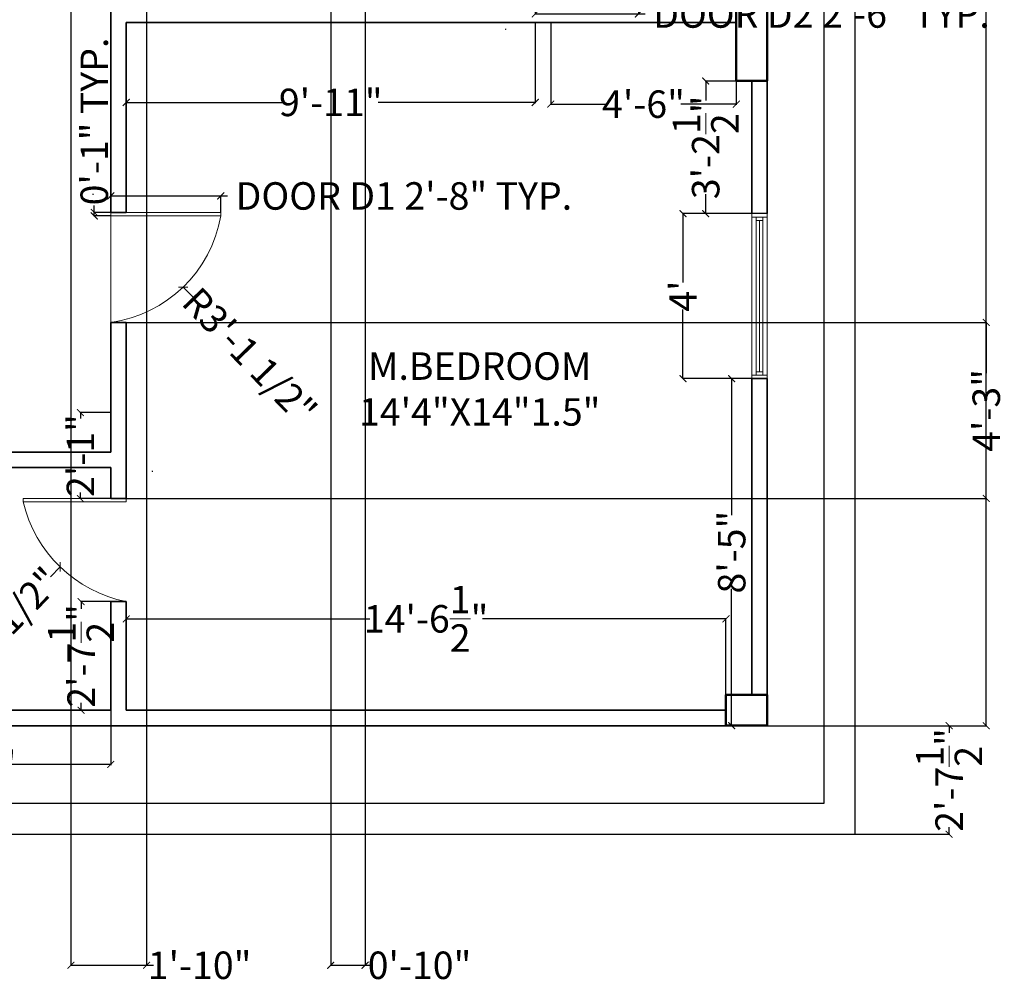
# Model space of a CAD drawing. Units: inches. Extents: x 490 to 1091, y 501 to 1322.
# Tile 2 of 5: x 804 to 1091, y 508 to 788. Entities that reach past the tile are written whole.
import ezdxf

# ---------------------------------------------------------------- set-up
doc = ezdxf.new("R2010")
doc.units = ezdxf.units.IN
doc.header["$MEASUREMENT"] = 0
for name, color, linetype, lineweight in [('A-ANNO-DIMS', 2, 'Continuous', 18), ('A-AREA-IDEN', 7, 'Continuous', 25), ('A-COLS', 12, 'Continuous', 50), ('A-DOOR', 3, 'Continuous', 20), ('A-GLAZ', 4, 'Continuous', 18), ('A-WALL', 7, 'Continuous', 35), ('C-PROP', 8, 'Continuous', 25)]:
    doc.layers.add(name, color=color, linetype=linetype, lineweight=lineweight)
doc.styles.get("Standard").update_dxf_attribs({"font": 'arial.ttf'})
doc.dimstyles.get("Standard").update_dxf_attribs({"dimtxt": 8, "dimasz": 2, "dimexe": 0.18, "dimexo": 0.0625, "dimgap": 0.09, "dimtad": 0, "dimdec": 1, "dimzin": 0, "dimdsep": 46, "dimlunit": 4, "dimtxsty": 'Standard', "dimblk": 'ARCHTICK', "dimcen": 0.09, "dimadec": 0, "dimazin": 0, "dimtfac": 1, "dimtdec": 1, "dimtofl": 0, "dimtmove": 0, "dimatfit": 3, "dimldrblk": 'ARCHTICK', "dimfxl": 1, "dimtolj": 1, "dimtzin": 0, "dimarcsym": 0})

# ---------------------------------------------------------------- blocks, each defined once
blk = doc.blocks.new('jcjg  bmvh')
for p, q in [((1232.66, 1066.6), (1223.66, 1066.6)), ((1223.66, 1066.6), (1223.66, 1042.6)), ((1232.66, 1042.6), (1232.66, 1066.6)), ((1223.66, 1042.6), (1232.66, 1042.6))]:
    blk.add_line(p, q)
blk = doc.blocks.new('bnfgfhvhm')
for p, q in [((1106.43, 1203.63), (1115.43, 1203.63)), ((1106.43, 1191.63), (1106.43, 1203.63)), ((1115.43, 1203.63), (1115.43, 1191.63)), ((1115.43, 1191.63), (1106.43, 1191.63))]:
    blk.add_line(p, q)
blk = doc.blocks.new('_ArchTick')
at = {"color": 0, "linetype": 'ByBlock', "const_width": 0.15}
blk.add_lwpolyline([(-0.5, -0.5), (0.5, 0.5)], dxfattribs=at)
blk = doc.blocks.new('*D16')
at = {"layer": 'A-ANNO-DIMS', "color": 0, "lineweight": -2, "transparency": 16777216}
for p, q in [((830.61, 618.58), (821.86, 618.58)), ((822.04, 618.58), (822.04, 616.49)), ((822.04, 586.98), (822.04, 589.08)), ((830.61, 586.98), (821.86, 586.98))]:
    blk.add_line(p, q, dxfattribs=at)
at = {"layer": 'Defpoints', "color": 0, "transparency": 16777216}
for p in [(822.04, 618.58), (830.67, 618.58), (830.67, 586.98)]:
    blk.add_point(p, dxfattribs=at)
at = {"layer": 'A-ANNO-DIMS', "color": 0, "lineweight": -2, "transparency": 16777216, "xscale": 2, "yscale": 2, "zscale": 2}
for p, rotation in [((822.04, 618.58), 90), ((822.04, 586.98), 270)]:
    blk.add_blockref('_ArchTick', p, dxfattribs=dict(at, rotation=rotation))
at = {"layer": 'A-ANNO-DIMS', "color": 0, "transparency": 16777216, "insert": (822.04, 602.78), "char_height": 8, "attachment_point": 5, "rotation": 90}
blk.add_mtext('\\A1;2\'-7{\\H1x;\\S1/2;}"', dxfattribs=at)
blk = doc.blocks.new('*D17')
at = {"layer": 'A-ANNO-DIMS', "color": 0, "lineweight": -2, "transparency": 16777216}
for p, q in [((830.61, 673.58), (821.66, 673.58)), ((821.84, 673.58), (821.84, 671.88)), ((830.61, 648.58), (821.66, 648.58)), ((821.84, 648.58), (821.84, 650.29))]:
    blk.add_line(p, q, dxfattribs=at)
at = {"layer": 'Defpoints', "color": 0, "transparency": 16777216}
for p in [(830.67, 673.58), (821.84, 648.58), (830.67, 648.58)]:
    blk.add_point(p, dxfattribs=at)
at = {"layer": 'A-ANNO-DIMS', "color": 0, "lineweight": -2, "transparency": 16777216, "xscale": 2, "yscale": 2, "zscale": 2}
for p, rotation in [((821.84, 673.58), 90), ((821.84, 648.58), 270)]:
    blk.add_blockref('_ArchTick', p, dxfattribs=dict(at, rotation=rotation))
at = {"layer": 'A-ANNO-DIMS', "color": 0, "transparency": 16777216, "insert": (821.84, 661.08), "char_height": 8, "attachment_point": 5, "rotation": 90}
blk.add_mtext('\\A1;2\'-1"', dxfattribs=at)
blk = doc.blocks.new('*D18')
at = {"layer": 'A-ANNO-DIMS', "color": 0, "lineweight": -2, "transparency": 16777216}
for p, q in [((751.67, 586.92), (751.67, 571.01)), ((830.67, 586.92), (830.67, 571.01)), ((751.67, 571.19), (780.42, 571.19)), ((830.67, 571.19), (801.91, 571.19))]:
    blk.add_line(p, q, dxfattribs=at)
at = {"layer": 'Defpoints', "color": 0, "transparency": 16777216}
for p in [(751.67, 586.98), (830.67, 586.98), (751.67, 571.19)]:
    blk.add_point(p, dxfattribs=at)
at = {"layer": 'A-ANNO-DIMS', "color": 0, "lineweight": -2, "transparency": 16777216, "xscale": 2, "yscale": 2, "zscale": 2, "rotation": 180}
blk.add_blockref('_ArchTick', (751.67, 571.19), dxfattribs=at)
at = {"layer": 'A-ANNO-DIMS', "color": 0, "lineweight": -2, "transparency": 16777216, "xscale": 2, "yscale": 2, "zscale": 2}
blk.add_blockref('_ArchTick', (830.67, 571.19), dxfattribs=at)
at = {"layer": 'A-ANNO-DIMS', "color": 0, "transparency": 16777216, "insert": (791.17, 571.19), "char_height": 8, "attachment_point": 5}
blk.add_mtext('\\A1;6\'-7"', dxfattribs=at)
blk = doc.blocks.new('mhjyhjykmjk')
for p, q in [((1017.17, 683.48), (1017.17, 731.48)), ((1017.17, 731.48), (1021.67, 731.48)), ((1021.67, 731.48), (1021.67, 683.48)), ((1017.17, 730.48), (1021.67, 730.48)), ((1018.42, 730.48), (1018.42, 684.48)), ((1018.42, 729.48), (1020.42, 729.48)), ((1019.42, 729.48), (1019.42, 685.48)), ((1020.42, 730.48), (1020.42, 684.48)), ((1020.42, 685.48), (1018.42, 685.48)), ((1021.67, 684.48), (1017.17, 684.48)), ((1021.67, 683.48), (1017.17, 683.48))]:
    blk.add_line(p, q)
at = {"layer": 'Defpoints'}
for p, q in [((1021.67, 731.48), (1017.17, 731.48)), ((1017.17, 683.48), (1021.67, 683.48))]:
    blk.add_line(p, q, dxfattribs=at)
blk = doc.blocks.new('*D37')
at = {"layer": 'A-ANNO-DIMS', "color": 0, "lineweight": -2, "transparency": 16777216}
for p, q in [((1021.73, 582.48), (1074.78, 582.48)), ((1074.6, 582.48), (1074.6, 580.39)), ((1074.6, 550.88), (1074.6, 552.98)), ((1047.33, 550.88), (1074.78, 550.88))]:
    blk.add_line(p, q, dxfattribs=at)
at = {"layer": 'Defpoints', "color": 0, "transparency": 16777216}
for p in [(1021.67, 582.48), (1047.27, 550.88), (1074.6, 550.88)]:
    blk.add_point(p, dxfattribs=at)
at = {"layer": 'A-ANNO-DIMS', "color": 0, "lineweight": -2, "transparency": 16777216, "xscale": 2, "yscale": 2, "zscale": 2}
for p, rotation in [((1074.6, 582.48), 90), ((1074.6, 550.88), 270)]:
    blk.add_blockref('_ArchTick', p, dxfattribs=dict(at, rotation=rotation))
at = {"layer": 'A-ANNO-DIMS', "color": 0, "transparency": 16777216, "insert": (1074.6, 566.68), "char_height": 8, "attachment_point": 5, "rotation": 90}
blk.add_mtext('\\A1;2\'-7{\\H1x;\\S1/2;}"', dxfattribs=at)
blk = doc.blocks.new('*D40')
at = {"layer": 'A-ANNO-DIMS', "color": 0, "lineweight": -2, "transparency": 16777216}
for p, q in [((835.17, 787.02), (835.17, 763.67)), ((954.17, 787.02), (954.17, 763.67)), ((835.17, 763.85), (880.84, 763.85)), ((954.17, 763.85), (908.5, 763.85))]:
    blk.add_line(p, q, dxfattribs=at)
at = {"layer": 'Defpoints', "color": 0, "transparency": 16777216}
for p in [(835.17, 787.08), (954.17, 787.08), (835.17, 763.85)]:
    blk.add_point(p, dxfattribs=at)
at = {"layer": 'A-ANNO-DIMS', "color": 0, "lineweight": -2, "transparency": 16777216, "xscale": 2, "yscale": 2, "zscale": 2, "rotation": 180}
blk.add_blockref('_ArchTick', (835.17, 763.85), dxfattribs=at)
at = {"layer": 'A-ANNO-DIMS', "color": 0, "lineweight": -2, "transparency": 16777216, "xscale": 2, "yscale": 2, "zscale": 2}
blk.add_blockref('_ArchTick', (954.17, 763.85), dxfattribs=at)
at = {"layer": 'A-ANNO-DIMS', "color": 0, "transparency": 16777216, "insert": (894.67, 763.85), "char_height": 8, "attachment_point": 5}
blk.add_mtext('\\A1;9\'-11"', dxfattribs=at)
blk = doc.blocks.new('*D41')
at = {"layer": 'A-ANNO-DIMS', "color": 0, "lineweight": -2, "transparency": 16777216}
for p, q in [((958.67, 787.02), (958.67, 763.17)), ((1012.67, 787.02), (1012.67, 763.17)), ((958.67, 763.35), (974.79, 763.35)), ((1012.67, 763.35), (996.55, 763.35))]:
    blk.add_line(p, q, dxfattribs=at)
at = {"layer": 'Defpoints', "color": 0, "transparency": 16777216}
for p in [(958.67, 787.08), (1012.67, 787.08), (1012.67, 763.35)]:
    blk.add_point(p, dxfattribs=at)
at = {"layer": 'A-ANNO-DIMS', "color": 0, "lineweight": -2, "transparency": 16777216, "xscale": 2, "yscale": 2, "zscale": 2, "rotation": 180}
blk.add_blockref('_ArchTick', (958.67, 763.35), dxfattribs=at)
at = {"layer": 'A-ANNO-DIMS', "color": 0, "lineweight": -2, "transparency": 16777216, "xscale": 2, "yscale": 2, "zscale": 2}
blk.add_blockref('_ArchTick', (1012.67, 763.35), dxfattribs=at)
at = {"layer": 'A-ANNO-DIMS', "color": 0, "transparency": 16777216, "insert": (985.67, 763.35), "char_height": 8, "attachment_point": 5}
blk.add_mtext('\\A1;4\'-6"', dxfattribs=at)
blk = doc.blocks.new('*D42')
at = {"layer": 'A-ANNO-DIMS', "color": 0, "lineweight": -2, "transparency": 16777216}
for p, q in [((1021.61, 683.48), (1011.14, 683.48)), ((1011.32, 683.48), (1011.32, 643.71)), ((1011.32, 582.48), (1011.32, 622.26)), ((1021.61, 582.48), (1011.14, 582.48))]:
    blk.add_line(p, q, dxfattribs=at)
at = {"layer": 'Defpoints', "color": 0, "transparency": 16777216}
for p in [(1021.67, 683.48), (1011.32, 582.48), (1021.67, 582.48)]:
    blk.add_point(p, dxfattribs=at)
at = {"layer": 'A-ANNO-DIMS', "color": 0, "lineweight": -2, "transparency": 16777216, "xscale": 2, "yscale": 2, "zscale": 2}
for p, rotation in [((1011.32, 683.48), 90), ((1011.32, 582.48), 270)]:
    blk.add_blockref('_ArchTick', p, dxfattribs=dict(at, rotation=rotation))
at = {"layer": 'A-ANNO-DIMS', "color": 0, "transparency": 16777216, "insert": (1011.32, 632.98), "char_height": 8, "attachment_point": 5, "rotation": 90}
blk.add_mtext('\\A1;8\'-5"', dxfattribs=at)
blk = doc.blocks.new('*D43')
at = {"layer": 'A-ANNO-DIMS', "color": 0, "lineweight": -2, "transparency": 16777216}
for p, q in [((1017.11, 731.48), (996.97, 731.48)), ((997.15, 731.48), (997.15, 711.42)), ((997.15, 683.48), (997.15, 703.55)), ((1017.11, 683.48), (996.97, 683.48))]:
    blk.add_line(p, q, dxfattribs=at)
at = {"layer": 'Defpoints', "color": 0, "transparency": 16777216}
for p in [(997.15, 731.48), (1017.17, 731.48), (1017.17, 683.48)]:
    blk.add_point(p, dxfattribs=at)
at = {"layer": 'A-ANNO-DIMS', "color": 0, "lineweight": -2, "transparency": 16777216, "xscale": 2, "yscale": 2, "zscale": 2}
for p, rotation in [((997.15, 731.48), 90), ((997.15, 683.48), 270)]:
    blk.add_blockref('_ArchTick', p, dxfattribs=dict(at, rotation=rotation))
at = {"layer": 'A-ANNO-DIMS', "color": 0, "transparency": 16777216, "insert": (997.15, 707.48), "char_height": 8, "attachment_point": 5, "rotation": 90}
blk.add_mtext("\\A1;4'", dxfattribs=at)
blk = doc.blocks.new('*D44')
at = {"layer": 'A-ANNO-DIMS', "color": 0, "lineweight": -2, "transparency": 16777216}
for p, q in [((1017.11, 770.08), (1003.58, 770.08)), ((1003.76, 770.08), (1003.76, 764.42)), ((1003.76, 731.48), (1003.76, 737.15)), ((1017.11, 731.48), (1003.58, 731.48))]:
    blk.add_line(p, q, dxfattribs=at)
at = {"layer": 'Defpoints', "color": 0, "transparency": 16777216}
for p in [(1017.17, 770.08), (1003.76, 731.48), (1017.17, 731.48)]:
    blk.add_point(p, dxfattribs=at)
at = {"layer": 'A-ANNO-DIMS', "color": 0, "lineweight": -2, "transparency": 16777216, "xscale": 2, "yscale": 2, "zscale": 2}
for p, rotation in [((1003.76, 770.08), 90), ((1003.76, 731.48), 270)]:
    blk.add_blockref('_ArchTick', p, dxfattribs=dict(at, rotation=rotation))
at = {"layer": 'A-ANNO-DIMS', "color": 0, "transparency": 16777216, "insert": (1003.76, 750.78), "char_height": 8, "attachment_point": 5, "rotation": 90}
blk.add_mtext('\\A1;3\'-2{\\H1x;\\S1/2;}"', dxfattribs=at)
blk = doc.blocks.new('*D45')
at = {"layer": 'A-ANNO-DIMS', "color": 0, "lineweight": -2, "transparency": 16777216}
for p, q in [((835.17, 587.05), (835.17, 613.75)), ((835.17, 613.57), (906.05, 613.57)), ((1009.67, 613.57), (938.79, 613.57)), ((1009.67, 587.05), (1009.67, 613.75))]:
    blk.add_line(p, q, dxfattribs=at)
at = {"layer": 'Defpoints', "color": 0, "transparency": 16777216}
for p in [(1009.67, 613.57), (835.17, 586.98), (1009.67, 586.98)]:
    blk.add_point(p, dxfattribs=at)
at = {"layer": 'A-ANNO-DIMS', "color": 0, "lineweight": -2, "transparency": 16777216, "xscale": 2, "yscale": 2, "zscale": 2, "rotation": 180}
blk.add_blockref('_ArchTick', (835.17, 613.57), dxfattribs=at)
at = {"layer": 'A-ANNO-DIMS', "color": 0, "lineweight": -2, "transparency": 16777216, "xscale": 2, "yscale": 2, "zscale": 2}
blk.add_blockref('_ArchTick', (1009.67, 613.57), dxfattribs=at)
at = {"layer": 'A-ANNO-DIMS', "color": 0, "transparency": 16777216, "insert": (922.42, 613.57), "char_height": 8, "attachment_point": 5}
blk.add_mtext('\\A1;14\'-6{\\H1x;\\S1/2;}"', dxfattribs=at)
blk = doc.blocks.new('DOOR-LEAF-32IN')
for p, q in [((-32, -1), (-32, 0)), ((-32, 0), (0, 0)), ((0, 0), (0, -1)), ((0, -1), (-32, -1))]:
    blk.add_line(p, q)
blk = doc.blocks.new('DOOR-LEAF-30IN')
for p, q in [((0, 0), (0, 1)), ((0, 1), (30, 1)), ((30, 0), (0, 0)), ((30, 1), (30, 0))]:
    blk.add_line(p, q)
blk = doc.blocks.new('*D54')
at = {"layer": 'A-ANNO-DIMS', "color": 0, "lineweight": -2, "transparency": 16777216}
for p, q in [((830.67, 731.9), (830.67, 736.81)), ((830.67, 736.63), (862.67, 736.63)), ((862.67, 731.9), (862.67, 736.81)), ((862.67, 736.63), (864.67, 736.63))]:
    blk.add_line(p, q, dxfattribs=at)
at = {"layer": 'Defpoints', "color": 0, "transparency": 16777216}
for p in [(862.67, 736.63), (830.67, 731.83), (862.67, 731.83)]:
    blk.add_point(p, dxfattribs=at)
at = {"layer": 'A-ANNO-DIMS', "color": 0, "lineweight": -2, "transparency": 16777216, "xscale": 2, "yscale": 2, "zscale": 2, "rotation": 180}
blk.add_blockref('_ArchTick', (830.67, 736.63), dxfattribs=at)
at = {"layer": 'A-ANNO-DIMS', "color": 0, "lineweight": -2, "transparency": 16777216, "xscale": 2, "yscale": 2, "zscale": 2}
blk.add_blockref('_ArchTick', (862.67, 736.63), dxfattribs=at)
at = {"layer": 'A-ANNO-DIMS', "color": 0, "transparency": 16777216, "insert": (915.95, 736.63), "char_height": 8, "attachment_point": 5}
blk.add_mtext('\\A1;DOOR D1 2\'-8" TYP.', dxfattribs=at)
blk = doc.blocks.new('*D55')
at = {"layer": 'A-ANNO-DIMS', "color": 0, "lineweight": -2, "transparency": 16777216}
for p, q in [((825.87, 731.83), (825.87, 733.83)), ((830.61, 731.83), (825.69, 731.83)), ((830.61, 730.83), (825.69, 730.83)), ((825.87, 730.83), (825.87, 731.83))]:
    blk.add_line(p, q, dxfattribs=at)
at = {"layer": 'Defpoints', "color": 0, "transparency": 16777216}
for p in [(825.87, 731.83), (830.67, 731.83), (830.67, 730.83)]:
    blk.add_point(p, dxfattribs=at)
at = {"layer": 'A-ANNO-DIMS', "color": 0, "lineweight": -2, "transparency": 16777216, "xscale": 2, "yscale": 2, "zscale": 2}
for p, rotation in [((825.87, 731.83), 90), ((825.87, 730.83), 270)]:
    blk.add_blockref('_ArchTick', p, dxfattribs=dict(at, rotation=rotation))
at = {"layer": 'A-ANNO-DIMS', "color": 0, "transparency": 16777216, "insert": (825.87, 758.3), "char_height": 8, "attachment_point": 5, "rotation": 90}
blk.add_mtext('\\A1;0\'-1" TYP.', dxfattribs=at)
blk = doc.blocks.new('*D56')
at = {"layer": 'A-ANNO-DIMS', "color": 0, "lineweight": -2, "transparency": 16777216}
for p, q in [((954.17, 794.02), (954.17, 789.4)), ((984.17, 794.02), (984.17, 789.4)), ((954.17, 789.58), (984.17, 789.58)), ((984.17, 789.58), (986.17, 789.58))]:
    blk.add_line(p, q, dxfattribs=at)
at = {"layer": 'Defpoints', "color": 0, "transparency": 16777216}
for p in [(954.17, 794.08), (984.17, 794.08), (984.17, 789.58)]:
    blk.add_point(p, dxfattribs=at)
at = {"layer": 'A-ANNO-DIMS', "color": 0, "lineweight": -2, "transparency": 16777216, "xscale": 2, "yscale": 2, "zscale": 2, "rotation": 180}
blk.add_blockref('_ArchTick', (954.17, 789.58), dxfattribs=at)
at = {"layer": 'A-ANNO-DIMS', "color": 0, "lineweight": -2, "transparency": 16777216, "xscale": 2, "yscale": 2, "zscale": 2}
blk.add_blockref('_ArchTick', (984.17, 789.58), dxfattribs=at)
at = {"layer": 'A-ANNO-DIMS', "color": 0, "transparency": 16777216, "insert": (1037.45, 789.58), "char_height": 8, "attachment_point": 5}
blk.add_mtext('\\A1;DOOR D2 2\'-6" TYP.', dxfattribs=at)
blk = doc.blocks.new('*D65')
at = {"layer": 'A-ANNO-DIMS', "color": 0, "lineweight": -2, "transparency": 16777216}
for p, q in [((1021.73, 1227.28), (1085.58, 1227.28)), ((1085.4, 1227.28), (1085.4, 918.72)), ((1085.4, 582.48), (1085.4, 891.05)), ((1021.73, 582.48), (1085.58, 582.48))]:
    blk.add_line(p, q, dxfattribs=at)
at = {"layer": 'Defpoints', "color": 0, "transparency": 16777216}
for p in [(1021.67, 1227.28), (1085.4, 1227.28), (1021.67, 582.48)]:
    blk.add_point(p, dxfattribs=at)
at = {"layer": 'A-ANNO-DIMS', "color": 0, "lineweight": -2, "transparency": 16777216, "xscale": 2, "yscale": 2, "zscale": 2}
for p, rotation in [((1085.4, 1227.28), 90), ((1085.4, 582.48), 270)]:
    blk.add_blockref('_ArchTick', p, dxfattribs=dict(at, rotation=rotation))
at = {"layer": 'A-ANNO-DIMS', "color": 0, "transparency": 16777216, "insert": (1085.4, 904.88), "char_height": 8, "attachment_point": 5, "rotation": 90}
blk.add_mtext('\\A1;53\'-9"', dxfattribs=at)
blk = doc.blocks.new('*D69')
at = {"layer": 'A-ANNO-DIMS', "color": 0, "lineweight": -2, "transparency": 16777216}
for p, q in [((894.67, 1182.97), (894.67, 512.57)), ((904.67, 1182.97), (904.67, 512.57)), ((894.67, 512.75), (904.67, 512.75)), ((904.67, 512.75), (906.67, 512.75))]:
    blk.add_line(p, q, dxfattribs=at)
at = {"layer": 'Defpoints', "color": 0, "transparency": 16777216}
for p in [(894.67, 1183.03), (904.67, 1183.03), (904.67, 512.75)]:
    blk.add_point(p, dxfattribs=at)
at = {"layer": 'A-ANNO-DIMS', "color": 0, "lineweight": -2, "transparency": 16777216, "xscale": 2, "yscale": 2, "zscale": 2, "rotation": 180}
blk.add_blockref('_ArchTick', (894.67, 512.75), dxfattribs=at)
at = {"layer": 'A-ANNO-DIMS', "color": 0, "lineweight": -2, "transparency": 16777216, "xscale": 2, "yscale": 2, "zscale": 2}
blk.add_blockref('_ArchTick', (904.67, 512.75), dxfattribs=at)
at = {"layer": 'A-ANNO-DIMS', "color": 0, "transparency": 16777216, "insert": (920.5, 512.75), "char_height": 8, "attachment_point": 5}
blk.add_mtext('\\A1;0\'-10"', dxfattribs=at)
blk = doc.blocks.new('*D71')
at = {"layer": 'A-ANNO-DIMS', "color": 0, "lineweight": -2, "transparency": 16777216}
for p, q in [((819.07, 1134.22), (819.07, 512.57)), ((841.07, 1134.22), (841.07, 512.57)), ((819.07, 512.75), (841.07, 512.75)), ((841.07, 512.75), (843.07, 512.75))]:
    blk.add_line(p, q, dxfattribs=at)
at = {"layer": 'Defpoints', "color": 0, "transparency": 16777216}
for p in [(819.07, 1134.28), (841.07, 1134.28), (841.07, 512.75)]:
    blk.add_point(p, dxfattribs=at)
at = {"layer": 'A-ANNO-DIMS', "color": 0, "lineweight": -2, "transparency": 16777216, "xscale": 2, "yscale": 2, "zscale": 2, "rotation": 180}
blk.add_blockref('_ArchTick', (819.07, 512.75), dxfattribs=at)
at = {"layer": 'A-ANNO-DIMS', "color": 0, "lineweight": -2, "transparency": 16777216, "xscale": 2, "yscale": 2, "zscale": 2}
blk.add_blockref('_ArchTick', (841.07, 512.75), dxfattribs=at)
at = {"layer": 'A-ANNO-DIMS', "color": 0, "transparency": 16777216, "insert": (856.52, 512.75), "char_height": 8, "attachment_point": 5}
blk.add_mtext('\\A1;1\'-10"', dxfattribs=at)
blk = doc.blocks.new('*D80')
at = {"layer": 'A-ANNO-DIMS', "color": 0, "lineweight": -2, "transparency": 16777216}
for p, q in [((830.73, 699.83), (1085.58, 699.83)), ((1085.4, 699.83), (1085.4, 685.09)), ((1085.4, 648.58), (1085.4, 663.32)), ((830.73, 648.58), (1085.58, 648.58))]:
    blk.add_line(p, q, dxfattribs=at)
at = {"layer": 'Defpoints', "color": 0, "transparency": 16777216}
for p in [(830.67, 699.83), (1085.4, 699.83), (830.67, 648.58)]:
    blk.add_point(p, dxfattribs=at)
at = {"layer": 'A-ANNO-DIMS', "color": 0, "lineweight": -2, "transparency": 16777216, "xscale": 2, "yscale": 2, "zscale": 2}
for p, rotation in [((1085.4, 699.83), 90), ((1085.4, 648.58), 270)]:
    blk.add_blockref('_ArchTick', p, dxfattribs=dict(at, rotation=rotation))
at = {"layer": 'A-ANNO-DIMS', "color": 0, "transparency": 16777216, "insert": (1085.4, 674.21), "char_height": 8, "attachment_point": 5, "rotation": 90}
blk.add_mtext('\\A1;4\'-3"', dxfattribs=at)
blk = doc.blocks.new('*D82')
at = {"layer": 'A-ANNO-DIMS', "color": 0, "lineweight": -2, "transparency": 16777216}
for p, q in [((979.77, 820.56), (973.27, 813.82)), ((945.48, 785.17), (945.66, 785.17)), ((945.57, 785.08), (945.57, 785.26))]:
    blk.add_line(p, q, dxfattribs=at)
at = {"layer": 'Defpoints', "color": 0, "transparency": 16777216}
for p in [(973.27, 813.82), (945.57, 785.17)]:
    blk.add_point(p, dxfattribs=at)
at = {"layer": 'A-ANNO-DIMS', "color": 0, "lineweight": -2, "transparency": 16777216, "xscale": 2, "yscale": 2, "zscale": 2, "rotation": 225.9717309641953}
blk.add_blockref('_ArchTick', (973.27, 813.82), dxfattribs=at)
at = {"layer": 'A-ANNO-DIMS', "color": 0, "transparency": 16777216, "insert": (989.89, 831.02), "char_height": 8, "attachment_point": 5, "rotation": 45.9717}
blk.add_mtext('\\A1;R3\'-4"', dxfattribs=at)
blk = doc.blocks.new('*D84')
at = {"layer": 'A-ANNO-DIMS', "color": 0, "lineweight": -2, "transparency": 16777216}
for p, q in [((842.73, 656.51), (842.91, 656.51)), ((842.82, 656.42), (842.82, 656.6)), ((813.15, 625.82), (815.93, 628.69))]:
    blk.add_line(p, q, dxfattribs=at)
at = {"layer": 'Defpoints', "color": 0, "transparency": 16777216}
for p in [(842.82, 656.51), (815.93, 628.69)]:
    blk.add_point(p, dxfattribs=at)
at = {"layer": 'A-ANNO-DIMS', "color": 0, "lineweight": -2, "transparency": 16777216, "xscale": 2, "yscale": 2, "zscale": 2, "rotation": 45.97167705914391}
blk.add_blockref('_ArchTick', (815.93, 628.69), dxfattribs=at)
at = {"layer": 'A-ANNO-DIMS', "color": 0, "transparency": 16777216, "insert": (796.55, 608.65), "char_height": 8, "attachment_point": 5, "rotation": 45.9717}
blk.add_mtext('\\A1;R3\'-2 1/2"', dxfattribs=at)
blk = doc.blocks.new('*D85')
at = {"layer": 'A-ANNO-DIMS', "color": 0, "lineweight": -2, "transparency": 16777216}
for p, q in [((825.42, 737.17), (825.6, 737.17)), ((825.51, 737.08), (825.51, 737.26)), ((854.52, 707.23), (851.74, 710.1))]:
    blk.add_line(p, q, dxfattribs=at)
at = {"layer": 'Defpoints', "color": 0, "transparency": 16777216}
for p in [(825.51, 737.17), (851.74, 710.1)]:
    blk.add_point(p, dxfattribs=at)
at = {"layer": 'A-ANNO-DIMS', "color": 0, "lineweight": -2, "transparency": 16777216, "xscale": 2, "yscale": 2, "zscale": 2, "rotation": 134.0898121406561}
blk.add_blockref('_ArchTick', (851.74, 710.1), dxfattribs=at)
at = {"layer": 'A-ANNO-DIMS', "color": 0, "transparency": 16777216, "insert": (871.13, 690.08), "char_height": 8, "attachment_point": 5, "rotation": 314.0898}
blk.add_mtext('\\A1;R3\'-1 1/2"', dxfattribs=at)

msp = doc.modelspace()

# ---------------------------------------------------------------- linework, layer by layer
at = {"layer": 'A-DOOR'}
msp.add_line((830.67, 731.83), (830.67, 699.83), dxfattribs=at)
for centre, radius, start, end in [((825.51, 737.17), 37.69, 277.8618, 350.3194), ((842.82, 656.51), 38.69, 193.3426, 258.5994)]:
    msp.add_arc(centre, radius, start, end, dxfattribs=at)
at = {"layer": 'A-WALL'}
for p, q in [((830.67, 731.83), (830.67, 794.08)), ((954.17, 787.08), (835.17, 787.08)), ((835.17, 731.83), (835.17, 787.08)), ((958.67, 787.08), (954.17, 787.08)), ((958.67, 787.08), (1012.67, 787.08)), ((1017.17, 770.08), (1017.17, 731.48)), ((1021.67, 770.08), (1021.67, 731.48)), ((830.67, 731.83), (835.17, 731.83)), ((830.67, 662.08), (830.67, 699.83)), ((835.17, 699.83), (830.67, 699.83)), ((835.17, 648.58), (835.17, 699.83)), ((1017.17, 683.48), (1017.17, 591.48)), ((1021.67, 683.48), (1021.67, 582.48)), ((830.67, 662.08), (830.67, 673.58)), ((706.57, 662.08), (830.67, 662.08)), ((711.07, 657.58), (830.67, 657.58)), ((830.67, 648.58), (830.67, 657.58)), ((830.67, 648.58), (830.67, 657.58)), ((830.67, 648.58), (835.17, 648.58)), ((830.67, 586.98), (830.67, 618.58)), ((830.67, 586.98), (830.67, 618.58)), ((830.67, 618.58), (835.17, 618.58)), ((835.17, 586.98), (835.17, 618.58)), ((751.67, 586.98), (830.67, 586.98)), ((835.17, 586.98), (1009.67, 586.98)), ((1021.67, 582.48), (751.67, 582.48))]:
    msp.add_line(p, q, dxfattribs=at)
at = {"layer": 'C-PROP'}
for p, q in [((1047.27, 550.88), (1047.27, 1270.88)), ((1038.27, 559.88), (1038.27, 1261.88)), ((576.27, 559.88), (1038.27, 559.88)), ((567.27, 550.88), (1047.27, 550.88))]:
    msp.add_line(p, q, dxfattribs=at)

# ---------------------------------------------------------------- block references
at = {"layer": 'A-COLS'}
msp.add_blockref('jcjg  bmvh', (-210.99, -272.51), dxfattribs=at)
at = {"layer": 'A-COLS', "rotation": 270}
msp.add_blockref('bnfgfhvhm', (-181.96, 1697.92), dxfattribs=at)
at = {"layer": 'A-DOOR'}
for name, p in [('DOOR-LEAF-32IN', (862.67, 731.83)), ('DOOR-LEAF-30IN', (805.17, 647.58))]:
    msp.add_blockref(name, p, dxfattribs=at)
at = {"layer": 'A-GLAZ'}
msp.add_blockref('mhjyhjykmjk', (0, 0), dxfattribs=at)

# ---------------------------------------------------------------- texts
at = {"layer": 'A-AREA-IDEN', "insert": (878.9, 691.12), "char_height": 8, "attachment_point": 1}
msp.add_mtext_dynamic_manual_height_columns('\\pxqc;M.BEDROOM\\P14\'4"X14"1.5"', width=118.2325, gutter_width=40, heights=[0], dxfattribs=at)

# ---------------------------------------------------------------- dimensions: what is measured, and where the dimension line sits
at = {"layer": 'A-ANNO-DIMS'}
for base, p1, p2, override, picture, middle in [((1085.4, 1227.28), (1021.67, 582.48), (1021.67, 1227.28), {"dimdec": 1, "dimlfac": 1, "dimrnd": 0, "dimzin": 1, "dimdsep": 46, "dimlunit": 4, "dimfrac": 2}, '*D65', (1085.4, 904.88)), ((1003.76, 731.48), (1017.17, 770.08), (1017.17, 731.48), {"dimclrd": 0, "dimclre": 0, "dimclrt": 0}, '*D44', (1003.76, 750.78)), ((997.15, 731.48), (1017.17, 683.48), (1017.17, 731.48), {"dimclrd": 0, "dimclre": 0, "dimclrt": 0}, '*D43', (997.15, 707.48)), ((1085.3998, 699.8325), (830.6698, 648.5848), (830.6698, 699.8325), {"dimdec": 1, "dimlfac": 1, "dimrnd": 0, "dimzin": 1, "dimdsep": 46, "dimlunit": 4, "dimfrac": 2}, '*D80', (1085.3998, 674.2086)), ((1011.32, 582.48), (1021.67, 683.48), (1021.67, 582.48), {"dimclrd": 0, "dimclre": 0, "dimclrt": 0}, '*D42', (1011.32, 632.98)), ((821.84, 648.58), (830.67, 673.58), (830.67, 648.58), {"dimclrd": 0, "dimclre": 0, "dimclrt": 0}, '*D17', (821.84, 661.08)), ((822.04, 618.58), (830.67, 586.98), (830.67, 618.58), {"dimclrd": 0, "dimclre": 0, "dimclrt": 0}, '*D16', (822.04, 602.78)), ((1074.6, 550.88), (1021.67, 582.48), (1047.27, 550.88), {"dimclrd": 0, "dimclre": 0, "dimclrt": 0}, '*D37', (1074.6, 566.68))]:
    dim = msp.add_linear_dim(base=base, p1=p1, p2=p2, angle=90, dimstyle='Standard', override=override, dxfattribs=at)
    dim.commit()
    dim.dimension.update_dxf_attribs({"geometry": picture, "text_midpoint": middle})
for base, p1, p2, override, picture, middle in [((904.67, 512.75), (894.67, 1183.03), (904.67, 1183.03), {"dimdec": 1, "dimlfac": 1, "dimrnd": 0, "dimzin": 1, "dimdsep": 46, "dimlunit": 4, "dimfrac": 2}, '*D69', (920.5, 512.75)), ((841.07, 512.75), (819.07, 1134.28), (841.07, 1134.28), {"dimdec": 1, "dimlfac": 1, "dimrnd": 0, "dimzin": 1, "dimdsep": 46, "dimlunit": 4, "dimfrac": 2}, '*D71', (856.52, 512.75)), ((835.17, 763.85), (954.17, 787.08), (835.17, 787.08), {"dimclrd": 0, "dimclre": 0, "dimclrt": 0}, '*D40', (894.67, 763.85)), ((1012.67, 763.35), (958.67, 787.08), (1012.67, 787.08), {"dimclrd": 0, "dimclre": 0, "dimclrt": 0}, '*D41', (985.67, 763.35)), ((1009.67, 613.57), (835.17, 586.98), (1009.67, 586.98), {"dimclrd": 0, "dimclre": 0, "dimclrt": 0}, '*D45', (922.42, 613.57)), ((751.67, 571.19), (830.67, 586.98), (751.67, 586.98), {"dimclrd": 0, "dimclre": 0, "dimclrt": 0}, '*D18', (791.17, 571.19))]:
    dim = msp.add_linear_dim(base=base, p1=p1, p2=p2, dimstyle='Standard', override=override, dxfattribs=at)
    dim.commit()
    dim.dimension.update_dxf_attribs({"geometry": picture, "text_midpoint": middle})
dim = msp.add_radius_dim(center=(945.57, 785.17), mpoint=(973.27, 813.82), dimstyle='Standard', override={"dimdec": 1, "dimlfac": 1, "dimrnd": 0, "dimzin": 1, "dimdsep": 46, "dimlunit": 4, "dimfrac": 2}, dxfattribs=at)
dim.commit()
dim.dimension.update_dxf_attribs({"geometry": '*D82', "text_midpoint": (989.89, 831.02), "dimtype": 164})
for base, p1, p2, text, picture, middle in [((984.17, 789.58), (954.17, 794.08), (984.17, 794.08), 'DOOR D2 <> TYP.', '*D56', (1037.45, 789.58)), ((862.67, 736.63), (830.67, 731.83), (862.67, 731.83), 'DOOR D1 <> TYP.', '*D54', (915.95, 736.63))]:
    dim = msp.add_linear_dim(base=base, p1=p1, p2=p2, text=text, dimstyle='Standard', override={"dimdec": 1, "dimlfac": 1, "dimrnd": 0, "dimzin": 1, "dimdsep": 46, "dimlunit": 4, "dimfrac": 2}, dxfattribs=at)
    dim.commit()
    dim.dimension.update_dxf_attribs({"geometry": picture, "text_midpoint": middle})
dim = msp.add_linear_dim(base=(825.87, 731.83), p1=(830.67, 730.83), p2=(830.67, 731.83), angle=90, text='<> TYP.', dimstyle='Standard', override={"dimdec": 1, "dimlfac": 1, "dimrnd": 0, "dimzin": 1, "dimdsep": 46, "dimlunit": 4, "dimfrac": 2}, dxfattribs=at)
dim.commit()
dim.dimension.update_dxf_attribs({"geometry": '*D55', "text_midpoint": (825.87, 758.3)})
for center, mpoint, picture, middle in [((825.51, 737.17), (851.74, 710.1), '*D85', (871.13, 690.08)), ((842.82, 656.51), (815.93, 628.69), '*D84', (796.55, 608.65))]:
    dim = msp.add_radius_dim(center=center, mpoint=mpoint, dimstyle='Standard', override={"dimdec": 1, "dimlfac": 1, "dimrnd": 0, "dimzin": 1, "dimdsep": 46, "dimlunit": 4, "dimfrac": 2}, dxfattribs=at)
    dim.commit()
    dim.dimension.update_dxf_attribs({"geometry": picture, "text_midpoint": middle})

doc.saveas('drawing.dxf')
